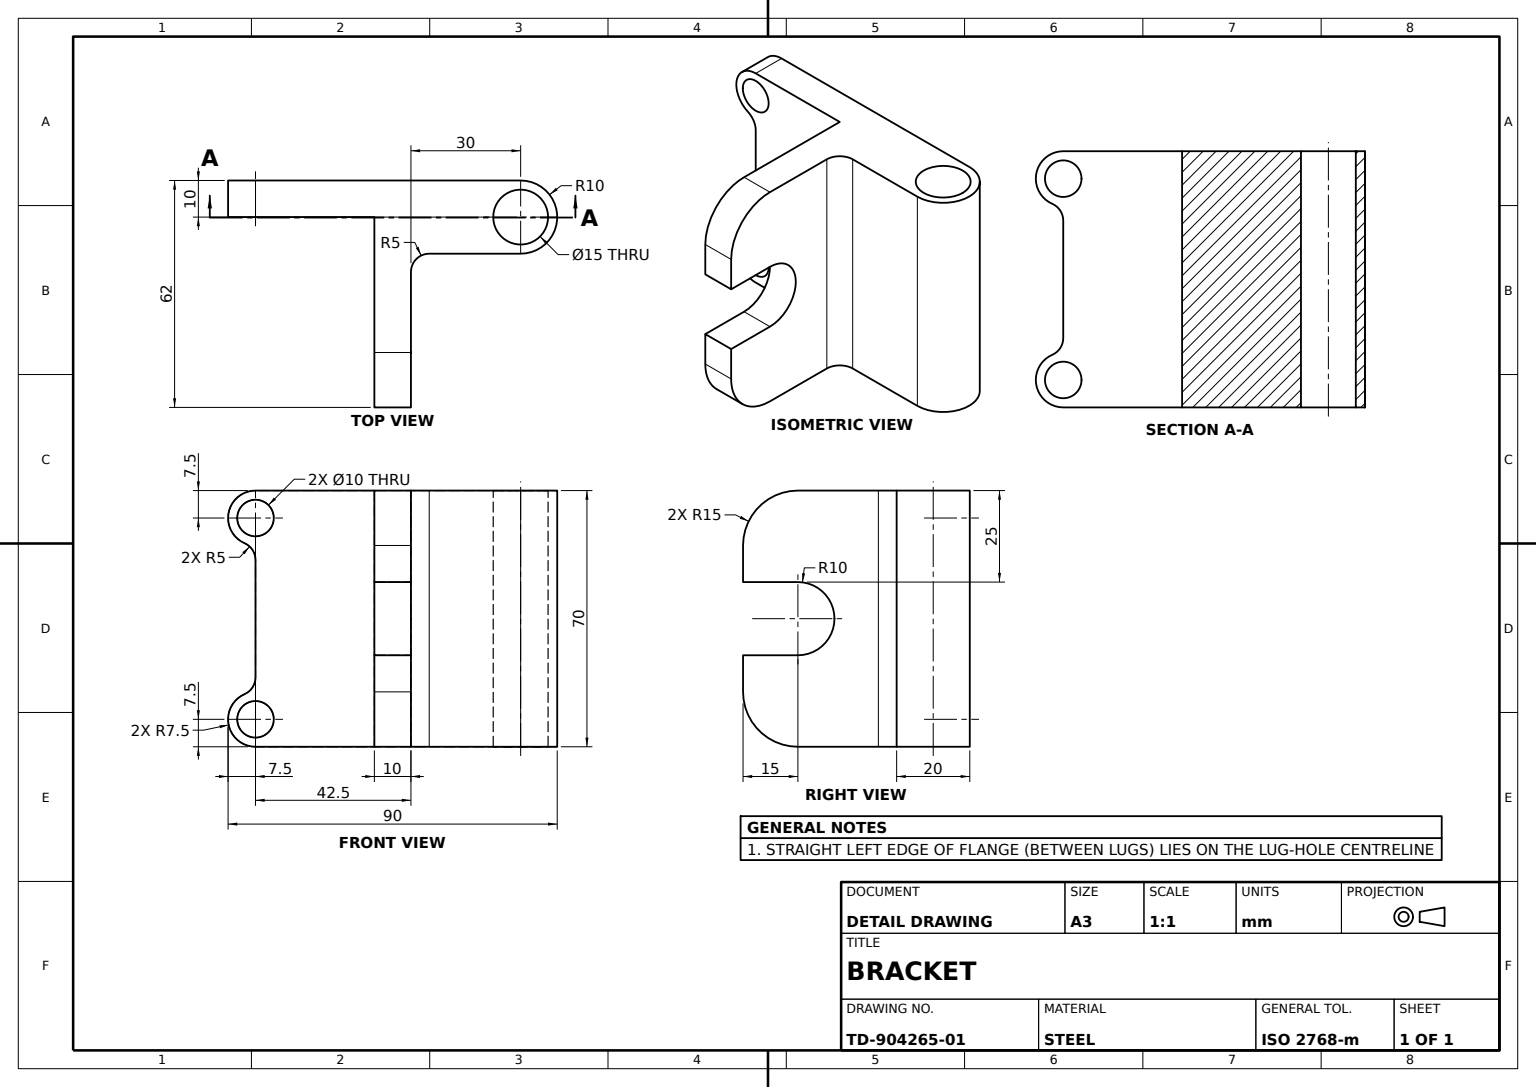
from build123d import *

# Parameters (mm, degrees)
BASE_PLATE_DEPTH         = 10
MOUNTING_FLANGE_SKETCH_W = 32.5
MOUNTING_FLANGE_SKETCH_H = 70
MOUNTING_FLANGE_DEPTH    = 10
FLANGE_LUGS_DEPTH        = 10
MOUNTING_HOLE_SKETCH_R   = 5
MOUNTING_HOLES_DEPTH     = 10
UPRIGHT_WEB_SKETCH_W     = 30
UPRIGHT_WEB_SKETCH_H     = 70
UPRIGHT_WEB_DEPTH        = 25
WEB_RELIEF_CUT_SKETCH_W  = 5
WEB_RELIEF_CUT_SKETCH_H  = 30
WEB_RELIEF_CUT_DEPTH     = 70
ROUNDED_ARM_DEPTH        = 70
BORE_BOSS_DEPTH          = 70
BORE_SKETCH_R            = 7.5
THROUGH_BORE_DEPTH       = 70


with BuildPart() as part:
    # Base Plate Sketch → Base Plate (new body)
    with BuildSketch(Plane.XY):
        with BuildLine():
            Line((0, 0), (47, 0))
            ThreePointArc((47, 0), (57.606601718, 4.393398282), (62, 15))
            Line((62, 15), (62, 25))
            Line((62, 25), (47, 25))
            ThreePointArc((47, 25), (37, 35), (47, 45))
            Line((47, 45), (62, 45))
            Line((62, 45), (62, 55))
            ThreePointArc((62, 55), (57.606601718, 65.606601718), (47, 70))
            Line((47, 70), (0, 70))
            Line((0, 70), (0, 0))
        make_face()
    extrude(amount=BASE_PLATE_DEPTH)

    # Mounting Flange Sketch → Mounting Flange (add)
    with BuildSketch(Plane.ZY):
        with Locations((26.25, 35)):
            Rectangle(MOUNTING_FLANGE_SKETCH_W, MOUNTING_FLANGE_SKETCH_H)
    extrude(amount=-MOUNTING_FLANGE_DEPTH)

    # Flange Lug Sketch → Flange Lugs (add)
    with BuildSketch(Plane(origin=(10, 0, 0), x_dir=(0, 0, -1), z_dir=(1, 0, 0))):
        with BuildLine():
            ThreePointArc((-45.5, 55.626136458), (-43.316699867, 53.78217355), (-42.5, 51.043560763))
            Line((-42.5, 51.043560763), (-42.5, 70))
            ThreePointArc((-42.5, 70), (-49.841797347, 64.032322328), (-45.5, 55.626136458))
        make_face()
        with BuildLine():
            Line((-42.5, 0), (-42.5, 18.956439237))
            ThreePointArc((-42.5, 18.956439237), (-43.316699867, 16.21782645), (-45.5, 14.373863542))
            ThreePointArc((-45.5, 14.373863542), (-49.841797347, 5.967677672), (-42.5, 0))
        make_face()
    extrude(amount=-FLANGE_LUGS_DEPTH)

    # Mounting Hole Sketch → Mounting Holes (cut)
    with BuildSketch(Plane(origin=(10, 0, 0), x_dir=(0, 0, -1), z_dir=(1, 0, 0))):
        with Locations((-42.5, 62.5)):
            Circle(MOUNTING_HOLE_SKETCH_R)
        with Locations((-42.5, 7.5)):
            Circle(MOUNTING_HOLE_SKETCH_R)
    extrude(amount=-MOUNTING_HOLES_DEPTH, mode=Mode.SUBTRACT)

    # Upright Web Sketch → Upright Web (add)
    with BuildSketch(Plane.ZY):
        with Locations((-15, 35)):
            Rectangle(UPRIGHT_WEB_SKETCH_W, UPRIGHT_WEB_SKETCH_H)
    extrude(amount=-UPRIGHT_WEB_DEPTH)

    # Web Relief Cut Sketch → Web Relief Cut (cut)
    with BuildSketch(Plane(origin=(0, 70, 0), x_dir=(1, 0, 0), z_dir=(0, 1, 0))):
        with Locations((22.5, 15)):
            Rectangle(WEB_RELIEF_CUT_SKETCH_W, WEB_RELIEF_CUT_SKETCH_H)
    extrude(amount=-WEB_RELIEF_CUT_DEPTH, mode=Mode.SUBTRACT)

    # Rounded Arm Sketch → Rounded Arm (add)
    with BuildSketch(Plane(origin=(0, 70, 0), x_dir=(1, 0, 0), z_dir=(0, 1, 0))):
        with BuildLine():
            Line((20, 0), (25, 0))
            ThreePointArc((25, 0), (21.464466094, 1.464466094), (20, 5))
            Line((20, 5), (20, 0))
        make_face()
    extrude(amount=-ROUNDED_ARM_DEPTH)

    # Bore Boss Sketch → Bore Boss (add)
    with BuildSketch(Plane(origin=(0, 70, 0), x_dir=(1, 0, 0), z_dir=(0, 1, 0))):
        with BuildLine():
            Line((0, 30), (20, 30))
            ThreePointArc((20, 30), (10, 40), (0, 30))
        make_face()
    extrude(amount=-BORE_BOSS_DEPTH)

    # Bore Sketch → Through Bore (cut)
    with BuildSketch(Plane(origin=(0, 70, 0), x_dir=(1, 0, 0), z_dir=(0, 1, 0))):
        with Locations(Location((10, 30, 0), (0, 0, 270))):
            Circle(BORE_SKETCH_R)
    extrude(amount=-THROUGH_BORE_DEPTH, mode=Mode.SUBTRACT)


solid = part.part
